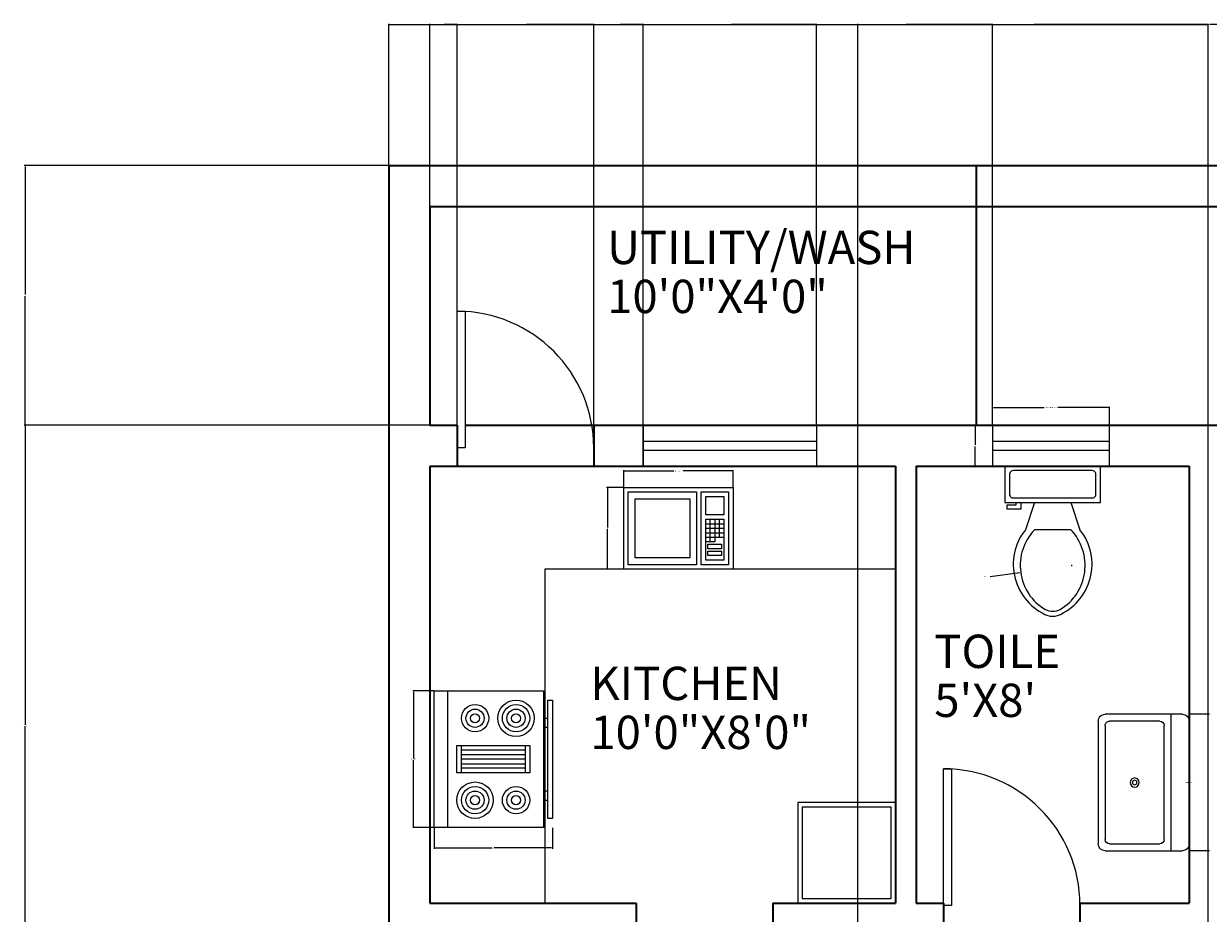
# Model space of a CAD drawing. Units: inches. Extents: x 25018 to 25490, y 41421 to 42101.
# Tile 3 of 5: x 25018 to 25279, y 41906 to 42101. Entities that reach past the tile are written whole.
import ezdxf

# ---------------------------------------------------------------- set-up
doc = ezdxf.new("R2010")
doc.units = ezdxf.units.IN
for name, color, linetype, lineweight in [('A-ANNO-DIMS', 2, 'Continuous', 18), ('A-AREA-IDEN', 7, 'Continuous', 18), ('A-DOOR', 3, 'Continuous', 25), ('A-EQPM', 8, 'Continuous', 18), ('A-FLOR-FIXT', 9, 'Continuous', 18), ('A-GLAZ', 4, 'Continuous', 18), ('A-WALL', 7, 'Continuous', 35)]:
    doc.layers.add(name, color=color, linetype=linetype, lineweight=lineweight)
doc.styles.get("Standard").update_dxf_attribs({"font": 'arial.ttf'})
doc.dimstyles.get("Standard").update_dxf_attribs({"dimtxt": 0.18, "dimasz": 0.18, "dimexe": 0.18, "dimexo": 0.0625, "dimgap": 0.09, "dimtad": 0, "dimtih": 1, "dimtoh": 1, "dimdec": 4, "dimzin": 0, "dimdsep": 46, "dimtxsty": 'Standard', "dimcen": 0.09, "dimadec": 0, "dimazin": 0, "dimtfac": 1, "dimtdec": 4, "dimtofl": 0, "dimtmove": 0, "dimatfit": 3, "dimfxl": 1, "dimtolj": 1, "dimtzin": 0, "dimarcsym": 0})

# ---------------------------------------------------------------- blocks, each defined once
blk = doc.blocks.new('*U2')
for p, q in [((0, 0), (0, -100)), ((750, 0), (750, -100))]:
    blk.add_line(p, q)
blk.add_lwpolyline([(0, 0), (0, 750), (43.75, 750), (43.75, 0)], close=True)
blk.add_arc((0, 0), 750, 0, 90)
blk = doc.blocks.new('Microwave')
for p, q in [((19, 7), (19, 11)), ((20, 11), (20, 7)), ((21, 7), (21, 11)), ((18, 10), (22, 10)), ((22, 9), (18, 9)), ((18, 8), (22, 8)), ((22, 7), (18, 7)), ((20, 6), (18, 6)), ((19, 6), (19, 7)), ((20, 7), (20, 6))]:
    blk.add_line(p, q)
for points in [[(0, 0), (0, 18), (24, 18), (24, 0)], [(1, 1), (1, 17), (16, 17), (16, 1)], [(17, 1), (17, 17), (23, 17), (23, 1)], [(18, 12), (18, 16), (22, 16), (22, 12)], [(2.5, 2.5), (2.5, 15.5), (14.5, 15.5), (14.5, 2.5)], [(18, 2), (18, 11), (22, 11), (22, 2)], [(18.5, 4.5), (18.5, 5.5), (21.5, 5.5), (21.5, 4.5)], [(18.5, 3), (18.5, 4), (21.5, 4), (21.5, 3)]]:
    blk.add_lwpolyline(points, close=True)
blk = doc.blocks.new('Range-Oven - 30 in top')
for p, q in [((0, -3), (30, -3)), ((12, -6), (18, -6)), ((13, -20), (13, -6)), ((14, -6), (14, -20)), ((15, -20), (15, -6)), ((16, -6), (16, -20)), ((17, -20), (17, -6)), ((18, -20), (12, -20)), ((6, -24), (6, -25)), ((8, -25), (8, -24)), ((22, -25), (22, -24)), ((24, -24), (24, -25))]:
    blk.add_line(p, q)
for points in [[(0, -24), (0, 0), (30, 0), (30, -24)], [(12, -21), (12, -5), (18, -5), (18, -21)], [(2, -26), (2, -25), (28, -25), (28, -26)]]:
    blk.add_lwpolyline(points, close=True)
for centre, radius in [((6, -9), 4), ((6, -9), 3), ((6, -9), 2), ((24, -9), 3), ((24, -9), 2), ((6, -9), 1), ((24, -9), 1), ((6, -18), 3), ((24, -18), 4), ((24, -18), 3), ((6, -18), 2), ((6, -18), 1), ((24, -18), 2), ((24, -18), 1)]:
    blk.add_circle(centre, radius)
blk = doc.blocks.new('Toilet - top')
for p, q in [((9.5, -6), (9.5, -2)), ((-10, -8.5), (-8, -8.5)), ((-10, -9.5), (-10, -8.5)), ((-7, -9.5), (-10, -9.5)), ((-8, -8.5), (-8, -8)), ((-7, -8), (-7, -9.5)), ((-4, -8), (-6, -14)), ((4, -8), (6, -14)), ((4, -14), (-4, -14))]:
    blk.add_line(p, q)
blk.add_lwpolyline([(10.5, -8), (10.5, 0), (-10.5, 0), (-10.5, -8)], close=True)
for points in [[(-9.5, -2), (-9.5, -6)], [(8.5, -1), (-8.5, -1)], [(-8.5, -7), (8.5, -7)]]:
    blk.add_lwpolyline(points)
for centre, radius, start, end in [((-8.62, -1.88), 0.884, 81.8699, 188.1301), ((8.62, -1.88), 0.884, 351.8699, 98.1301), ((-8.62, -6.12), 0.884, 171.8699, 278.1301), ((8.62, -6.12), 0.884, 261.8699, 8.1301), ((3.52, -21.58), 12.17, 141.4691, 247.9714), ((4.2, -21.82), 11.33, 136.3677, 238.9468), ((-3.52, -21.58), 12.17, 292.0284, 38.5307), ((-4.2, -21.82), 11.33, 301.053, 43.6321), ((0, -27.88), 4, 245.7318, 294.2682), ((0, -29), 4, 254.8605, 285.1395)]:
    blk.add_arc(centre, radius, start, end)
blk = doc.blocks.new('Sink-single - 30 in top')
blk.add_line((-15, -3.999996), (15, -3.999996))
for points in [[(-13.5, 0), (13.5, 0)], [(-15, -18.499996), (-15, -1.5)], [(15, -1.5), (15, -18.499996)], [(-13.5, -17.499996), (-13.5, -6.499996)], [(-12.5, -5.499996), (12.5, -5.499996)], [(13.5, -6.499996), (13.5, -17.499996)], [(13.5, -19.999996), (-13.5, -19.999996)], [(12.5, -18.499996), (-12.5, -18.499996)]]:
    blk.add_lwpolyline(points)
for radius in [1, 0.5]:
    blk.add_circle((0, -11.999996), radius)
for centre, radius, start, end in [((-13.5, -1.5), 1.5, 90, 180), ((13.5, -1.5), 1.5, 0, 90), ((-12.5, -6.499996), 1, 90, 180), ((12.5, -6.499996), 1, 0, 90), ((-12.5, -17.499996), 1, 180, 270), ((12.5, -17.499996), 1, 270, 0), ((-13.5, -18.499996), 1.5, 180, 270), ((13.5, -18.499996), 1.5, 270, 0)]:
    blk.add_arc(centre, radius, start, end)
blk = doc.blocks.new('WIN-BATH')
for p, q in [((0, 9), (0, 0)), ((25.67, 0), (25.67, 9)), ((0, 5.5), (25.67, 5.5)), ((0, 3.5), (25.67, 3.5))]:
    blk.add_line(p, q)
blk = doc.blocks.new('*D30')
at = {"layer": 'A-ANNO-DIMS', "color": 0, "lineweight": -2, "transparency": 16777216}
for p, q in [((25278.89, 41949.53), (25274.27, 41949.53)), ((25274.45, 41949.35), (25274.45, 41934.71)), ((25274.45, 41919.71), (25274.45, 41934.35)), ((25278.89, 41919.53), (25274.27, 41919.53))]:
    blk.add_line(p, q, dxfattribs=at)
at = {"layer": 'A-ANNO-DIMS', "color": 0, "transparency": 16777216}
for points in [[(25274.42, 41949.35), (25274.48, 41949.35), (25274.45, 41949.53)], [(25274.42, 41919.71), (25274.48, 41919.71), (25274.45, 41919.53)]]:
    blk.add_solid(points, dxfattribs=at)
at = {"layer": 'Defpoints', "color": 0, "transparency": 16777216}
for p in [(25274.45, 41949.53), (25278.95, 41949.53), (25278.95, 41919.53)]:
    blk.add_point(p, dxfattribs=at)
at = {"layer": 'A-ANNO-DIMS', "color": 0, "transparency": 16777216, "insert": (25274.45, 41934.53), "char_height": 0.18, "attachment_point": 5}
blk.add_mtext('\\A1;BASIN 30 TYP.', dxfattribs=at)
blk = doc.blocks.new('*D32')
at = {"layer": 'A-ANNO-DIMS', "color": 0, "lineweight": -2, "transparency": 16777216}
for p, q in [((25231.25, 42013.11), (25231.25, 42017.08)), ((25231.43, 42016.9), (25242.6, 42016.9)), ((25256.74, 42016.9), (25245.57, 42016.9)), ((25256.92, 42013.11), (25256.92, 42017.08))]:
    blk.add_line(p, q, dxfattribs=at)
at = {"layer": 'A-ANNO-DIMS', "color": 0, "transparency": 16777216}
for points in [[(25231.43, 42016.93), (25231.43, 42016.87), (25231.25, 42016.9)], [(25256.74, 42016.93), (25256.74, 42016.87), (25256.92, 42016.9)]]:
    blk.add_solid(points, dxfattribs=at)
at = {"layer": 'Defpoints', "color": 0, "transparency": 16777216}
for p in [(25256.92, 42016.9), (25231.25, 42013.05), (25256.92, 42013.05)]:
    blk.add_point(p, dxfattribs=at)
at = {"layer": 'A-ANNO-DIMS', "color": 0, "transparency": 16777216, "insert": (25244.09, 42016.9), "char_height": 0.18, "attachment_point": 5}
blk.add_mtext('\\A1;BATH WINDOW 26 TYP.', dxfattribs=at)
blk = doc.blocks.new('*D33')
at = {"layer": 'A-ANNO-DIMS', "color": 0, "lineweight": -2, "transparency": 16777216}
for p, q in [((25231.19, 42013.05), (25227.22, 42013.05)), ((25227.4, 42012.87), (25227.4, 42008.73)), ((25227.4, 42004.23), (25227.4, 42008.37)), ((25231.19, 42004.05), (25227.22, 42004.05))]:
    blk.add_line(p, q, dxfattribs=at)
at = {"layer": 'A-ANNO-DIMS', "color": 0, "transparency": 16777216}
for points in [[(25227.37, 42012.87), (25227.43, 42012.87), (25227.4, 42013.05)], [(25227.37, 42004.23), (25227.43, 42004.23), (25227.4, 42004.05)]]:
    blk.add_solid(points, dxfattribs=at)
at = {"layer": 'Defpoints', "color": 0, "transparency": 16777216}
for p in [(25227.4, 42013.05), (25231.25, 42013.05), (25231.25, 42004.05)]:
    blk.add_point(p, dxfattribs=at)
at = {"layer": 'A-ANNO-DIMS', "color": 0, "transparency": 16777216, "insert": (25227.4, 42008.55), "char_height": 0.18, "attachment_point": 5}
blk.add_mtext('\\A1;9 TYP.', dxfattribs=at)
blk = doc.blocks.new('*D34')
at = {"layer": 'A-ANNO-DIMS', "color": 0, "lineweight": -2, "transparency": 16777216}
for p, q in [((25150.25, 41999.43), (25150.25, 42003.15)), ((25150.43, 42002.97), (25161.21, 42002.97)), ((25174.07, 42002.97), (25163.29, 42002.97)), ((25174.25, 41999.43), (25174.25, 42003.15))]:
    blk.add_line(p, q, dxfattribs=at)
at = {"layer": 'A-ANNO-DIMS', "color": 0, "transparency": 16777216}
for points in [[(25150.43, 42003), (25150.43, 42002.94), (25150.25, 42002.97)], [(25174.07, 42003), (25174.07, 42002.94), (25174.25, 42002.97)]]:
    blk.add_solid(points, dxfattribs=at)
at = {"layer": 'Defpoints', "color": 0, "transparency": 16777216}
for p in [(25174.25, 42002.97), (25150.25, 41999.37), (25174.25, 41999.37)]:
    blk.add_point(p, dxfattribs=at)
at = {"layer": 'A-ANNO-DIMS', "color": 0, "transparency": 16777216, "insert": (25162.25, 42002.97), "char_height": 0.18, "attachment_point": 5}
blk.add_mtext('\\A1;MICROWAVE 24', dxfattribs=at)
blk = doc.blocks.new('*D35')
at = {"layer": 'A-ANNO-DIMS', "color": 0, "lineweight": -2, "transparency": 16777216}
for p, q in [((25150.19, 41999.37), (25146.47, 41999.37)), ((25146.65, 41999.19), (25146.65, 41990.55)), ((25146.65, 41981.55), (25146.65, 41990.19)), ((25150.19, 41981.37), (25146.47, 41981.37))]:
    blk.add_line(p, q, dxfattribs=at)
at = {"layer": 'A-ANNO-DIMS', "color": 0, "transparency": 16777216}
for points in [[(25146.62, 41999.19), (25146.68, 41999.19), (25146.65, 41999.37)], [(25146.62, 41981.55), (25146.68, 41981.55), (25146.65, 41981.37)]]:
    blk.add_solid(points, dxfattribs=at)
at = {"layer": 'Defpoints', "color": 0, "transparency": 16777216}
for p in [(25146.65, 41999.37), (25150.25, 41999.37), (25150.25, 41981.37)]:
    blk.add_point(p, dxfattribs=at)
at = {"layer": 'A-ANNO-DIMS', "color": 0, "transparency": 16777216, "insert": (25146.65, 41990.37), "char_height": 0.18, "attachment_point": 5}
blk.add_mtext('\\A1;18', dxfattribs=at)
blk = doc.blocks.new('*D36')
at = {"layer": 'A-ANNO-DIMS', "color": 0, "lineweight": -2, "transparency": 16777216}
for p, q in [((25108.53, 41954.65), (25103.91, 41954.65)), ((25104.09, 41954.47), (25104.09, 41939.84)), ((25104.09, 41924.83), (25104.09, 41939.47)), ((25108.53, 41924.65), (25103.91, 41924.65))]:
    blk.add_line(p, q, dxfattribs=at)
at = {"layer": 'A-ANNO-DIMS', "color": 0, "transparency": 16777216}
for points in [[(25104.06, 41954.47), (25104.12, 41954.47), (25104.09, 41954.65)], [(25104.06, 41924.83), (25104.12, 41924.83), (25104.09, 41924.65)]]:
    blk.add_solid(points, dxfattribs=at)
at = {"layer": 'Defpoints', "color": 0, "transparency": 16777216}
for p in [(25104.09, 41954.65), (25108.59, 41954.65), (25108.59, 41924.65)]:
    blk.add_point(p, dxfattribs=at)
at = {"layer": 'A-ANNO-DIMS', "color": 0, "transparency": 16777216, "insert": (25104.09, 41939.65), "char_height": 0.18, "attachment_point": 5}
blk.add_mtext('\\A1;RANGE 30', dxfattribs=at)
blk = doc.blocks.new('*D37')
at = {"layer": 'A-ANNO-DIMS', "color": 0, "lineweight": -2, "transparency": 16777216}
for p, q in [((25108.59, 41924.59), (25108.59, 41919.97)), ((25134.59, 41924.59), (25134.59, 41919.97)), ((25108.77, 41920.15), (25121.37, 41920.15)), ((25134.41, 41920.15), (25121.81, 41920.15))]:
    blk.add_line(p, q, dxfattribs=at)
at = {"layer": 'A-ANNO-DIMS', "color": 0, "transparency": 16777216}
for points in [[(25108.77, 41920.18), (25108.77, 41920.12), (25108.59, 41920.15)], [(25134.41, 41920.18), (25134.41, 41920.12), (25134.59, 41920.15)]]:
    blk.add_solid(points, dxfattribs=at)
at = {"layer": 'Defpoints', "color": 0, "transparency": 16777216}
for p in [(25108.59, 41924.65), (25134.59, 41924.65), (25108.59, 41920.15)]:
    blk.add_point(p, dxfattribs=at)
at = {"layer": 'A-ANNO-DIMS', "color": 0, "transparency": 16777216, "insert": (25121.59, 41920.15), "char_height": 0.18, "attachment_point": 5}
blk.add_mtext('\\A1;26', dxfattribs=at)
blk = doc.blocks.new('*D38')
at = {"layer": 'A-ANNO-DIMS', "color": 0, "lineweight": -2, "transparency": 16777216}
for p, q in [((25098.65, 42070.11), (25098.65, 42101.23)), ((25098.83, 42101.05), (25278.36, 42101.05)), ((25458.47, 42101.05), (25278.94, 42101.05)), ((25458.65, 42070.11), (25458.65, 42101.23))]:
    blk.add_line(p, q, dxfattribs=at)
at = {"layer": 'A-ANNO-DIMS', "color": 0, "transparency": 16777216}
for points in [[(25098.83, 42101.08), (25098.83, 42101.02), (25098.65, 42101.05)], [(25458.47, 42101.08), (25458.47, 42101.02), (25458.65, 42101.05)]]:
    blk.add_solid(points, dxfattribs=at)
at = {"layer": 'Defpoints', "color": 0, "transparency": 16777216}
for p in [(25458.65, 42101.05), (25098.65, 42070.05), (25458.65, 42070.05)]:
    blk.add_point(p, dxfattribs=at)
at = {"layer": 'A-ANNO-DIMS', "color": 0, "transparency": 16777216, "insert": (25278.65, 42101.05), "char_height": 0.18, "attachment_point": 5}
blk.add_mtext('\\A1;360', dxfattribs=at)
blk = doc.blocks.new('*D48')
at = {"layer": 'A-ANNO-DIMS', "color": 0, "lineweight": -2, "transparency": 16777216}
for p, q in [((25107.59, 42013.05), (25018.58, 42013.05)), ((25018.76, 42012.87), (25018.76, 41947.18)), ((25018.76, 41881.12), (25018.76, 41946.81)), ((25098.59, 41880.94), (25018.58, 41880.94))]:
    blk.add_line(p, q, dxfattribs=at)
at = {"layer": 'A-ANNO-DIMS', "color": 0, "transparency": 16777216}
for points in [[(25018.73, 42012.87), (25018.79, 42012.87), (25018.76, 42013.05)], [(25018.73, 41881.12), (25018.79, 41881.12), (25018.76, 41880.94)]]:
    blk.add_solid(points, dxfattribs=at)
at = {"layer": 'Defpoints', "color": 0, "transparency": 16777216}
for p in [(25018.76, 42013.05), (25107.65, 42013.05), (25098.65, 41880.94)]:
    blk.add_point(p, dxfattribs=at)
at = {"layer": 'A-ANNO-DIMS', "color": 0, "transparency": 16777216, "insert": (25018.76, 41946.99), "char_height": 0.18, "attachment_point": 5}
blk.add_mtext('\\A1;132.1', dxfattribs=at)
blk = doc.blocks.new('*D49')
at = {"layer": 'A-ANNO-DIMS', "color": 0, "lineweight": -2, "transparency": 16777216}
for p, q in [((25098.59, 42070.05), (25018.58, 42070.05)), ((25018.76, 42069.87), (25018.76, 42041.73)), ((25018.76, 42013.23), (25018.76, 42041.37)), ((25107.59, 42013.05), (25018.58, 42013.05))]:
    blk.add_line(p, q, dxfattribs=at)
at = {"layer": 'A-ANNO-DIMS', "color": 0, "transparency": 16777216}
for points in [[(25018.73, 42069.87), (25018.79, 42069.87), (25018.76, 42070.05)], [(25018.73, 42013.23), (25018.79, 42013.23), (25018.76, 42013.05)]]:
    blk.add_solid(points, dxfattribs=at)
at = {"layer": 'Defpoints', "color": 0, "transparency": 16777216}
for p in [(25018.76, 42070.05), (25098.65, 42070.05), (25107.65, 42013.05)]:
    blk.add_point(p, dxfattribs=at)
at = {"layer": 'A-ANNO-DIMS', "color": 0, "transparency": 16777216, "insert": (25018.76, 42041.55), "char_height": 0.18, "attachment_point": 5}
blk.add_mtext('\\A1;57', dxfattribs=at)
blk = doc.blocks.new('*D59')
at = {"layer": 'A-ANNO-DIMS', "color": 0, "lineweight": -2, "transparency": 16777216}
for p, q in [((25107.652612, 42013.112335), (25107.652612, 42101.229835)), ((25107.832612, 42101.049835), (25110.503185, 42101.049835)), ((25113.472612, 42101.049835), (25110.802039, 42101.049835)), ((25113.652612, 42013.112335), (25113.652612, 42101.229835))]:
    blk.add_line(p, q, dxfattribs=at)
at = {"layer": 'A-ANNO-DIMS', "color": 0, "transparency": 16777216}
for points in [[(25107.832612, 42101.079835), (25107.832612, 42101.019835), (25107.652612, 42101.049835)], [(25113.472612, 42101.079835), (25113.472612, 42101.019835), (25113.652612, 42101.049835)]]:
    blk.add_solid(points, dxfattribs=at)
at = {"layer": 'Defpoints', "color": 0, "transparency": 16777216}
for p in [(25113.652612, 42101.049835), (25107.652612, 42013.049835), (25113.652612, 42013.049835)]:
    blk.add_point(p, dxfattribs=at)
at = {"layer": 'A-ANNO-DIMS', "color": 0, "transparency": 16777216, "insert": (25110.652612, 42101.049835), "char_height": 0.18, "attachment_point": 5}
blk.add_mtext('\\A1;6', dxfattribs=at)
blk = doc.blocks.new('*D60')
at = {"layer": 'A-ANNO-DIMS', "color": 0, "lineweight": -2, "transparency": 16777216}
for p, q in [((25113.65, 42013.11), (25113.65, 42101.23)), ((25113.83, 42101.05), (25128.43, 42101.05)), ((25143.47, 42101.05), (25128.87, 42101.05)), ((25143.65, 42013.11), (25143.65, 42101.23))]:
    blk.add_line(p, q, dxfattribs=at)
at = {"layer": 'A-ANNO-DIMS', "color": 0, "transparency": 16777216}
for points in [[(25113.83, 42101.08), (25113.83, 42101.02), (25113.65, 42101.05)], [(25143.47, 42101.08), (25143.47, 42101.02), (25143.65, 42101.05)]]:
    blk.add_solid(points, dxfattribs=at)
at = {"layer": 'Defpoints', "color": 0, "transparency": 16777216}
for p in [(25143.65, 42101.05), (25113.65, 42013.05), (25143.65, 42013.05)]:
    blk.add_point(p, dxfattribs=at)
at = {"layer": 'A-ANNO-DIMS', "color": 0, "transparency": 16777216, "insert": (25128.65, 42101.05), "char_height": 0.18, "attachment_point": 5}
blk.add_mtext('\\A1;30', dxfattribs=at)
blk = doc.blocks.new('*D61')
at = {"layer": 'A-ANNO-DIMS', "color": 0, "lineweight": -2, "transparency": 16777216}
for p, q in [((25143.65, 42013.11), (25143.65, 42101.23)), ((25143.83, 42101.05), (25148.62, 42101.05)), ((25154.32, 42101.05), (25149.53, 42101.05)), ((25154.5, 42013.11), (25154.5, 42101.23))]:
    blk.add_line(p, q, dxfattribs=at)
at = {"layer": 'A-ANNO-DIMS', "color": 0, "transparency": 16777216}
for points in [[(25143.83, 42101.08), (25143.83, 42101.02), (25143.65, 42101.05)], [(25154.32, 42101.08), (25154.32, 42101.02), (25154.5, 42101.05)]]:
    blk.add_solid(points, dxfattribs=at)
at = {"layer": 'Defpoints', "color": 0, "transparency": 16777216}
for p in [(25154.5, 42101.05), (25143.65, 42013.05), (25154.5, 42013.05)]:
    blk.add_point(p, dxfattribs=at)
at = {"layer": 'A-ANNO-DIMS', "color": 0, "transparency": 16777216, "insert": (25149.08, 42101.05), "char_height": 0.18, "attachment_point": 5}
blk.add_mtext('\\A1;10.849', dxfattribs=at)
blk = doc.blocks.new('*D62')
at = {"layer": 'A-ANNO-DIMS', "color": 0, "lineweight": -2, "transparency": 16777216}
for p, q in [((25154.5, 42013.11), (25154.5, 42101.23)), ((25154.68, 42101.05), (25173.14, 42101.05)), ((25192.38, 42101.05), (25173.93, 42101.05)), ((25192.56, 42013.11), (25192.56, 42101.23))]:
    blk.add_line(p, q, dxfattribs=at)
at = {"layer": 'A-ANNO-DIMS', "color": 0, "transparency": 16777216}
for points in [[(25154.68, 42101.08), (25154.68, 42101.02), (25154.5, 42101.05)], [(25192.38, 42101.08), (25192.38, 42101.02), (25192.56, 42101.05)]]:
    blk.add_solid(points, dxfattribs=at)
at = {"layer": 'Defpoints', "color": 0, "transparency": 16777216}
for p in [(25192.56, 42101.05), (25154.5, 42013.05), (25192.56, 42013.05)]:
    blk.add_point(p, dxfattribs=at)
at = {"layer": 'A-ANNO-DIMS', "color": 0, "transparency": 16777216, "insert": (25173.53, 42101.05), "char_height": 0.18, "attachment_point": 5}
blk.add_mtext('\\A1;38.06', dxfattribs=at)
blk = doc.blocks.new('*D63')
at = {"layer": 'A-ANNO-DIMS', "color": 0, "lineweight": -2, "transparency": 16777216}
for p, q in [((25192.56, 42013.11), (25192.56, 42101.23)), ((25192.74, 42101.05), (25211.51, 42101.05)), ((25231.07, 42101.05), (25212.3, 42101.05)), ((25231.25, 42013.11), (25231.25, 42101.23))]:
    blk.add_line(p, q, dxfattribs=at)
at = {"layer": 'A-ANNO-DIMS', "color": 0, "transparency": 16777216}
for points in [[(25192.74, 42101.08), (25192.74, 42101.02), (25192.56, 42101.05)], [(25231.07, 42101.08), (25231.07, 42101.02), (25231.25, 42101.05)]]:
    blk.add_solid(points, dxfattribs=at)
at = {"layer": 'Defpoints', "color": 0, "transparency": 16777216}
for p in [(25231.25, 42101.05), (25192.56, 42013.05), (25231.25, 42013.05)]:
    blk.add_point(p, dxfattribs=at)
at = {"layer": 'A-ANNO-DIMS', "color": 0, "transparency": 16777216, "insert": (25211.91, 42101.05), "char_height": 0.18, "attachment_point": 5}
blk.add_mtext('\\A1;38.69', dxfattribs=at)
blk = doc.blocks.new('*D75')
at = {"layer": 'A-ANNO-DIMS', "color": 0, "lineweight": -2, "transparency": 16777216}
for p, q in [((25201.64, 41804.94), (25201.64, 42101.23)), ((25201.82, 42101.05), (25239.92, 42101.05)), ((25278.45, 42101.05), (25240.36, 42101.05)), ((25278.63, 41804.94), (25278.63, 42101.23))]:
    blk.add_line(p, q, dxfattribs=at)
at = {"layer": 'A-ANNO-DIMS', "color": 0, "transparency": 16777216}
for points in [[(25201.82, 42101.08), (25201.82, 42101.02), (25201.64, 42101.05)], [(25278.45, 42101.08), (25278.45, 42101.02), (25278.63, 42101.05)]]:
    blk.add_solid(points, dxfattribs=at)
at = {"layer": 'Defpoints', "color": 0, "transparency": 16777216}
for p in [(25278.63, 42101.05), (25201.64, 41804.88), (25278.63, 41804.88)]:
    blk.add_point(p, dxfattribs=at)
at = {"layer": 'A-ANNO-DIMS', "color": 0, "transparency": 16777216, "insert": (25240.14, 42101.05), "char_height": 0.18, "attachment_point": 5}
blk.add_mtext('\\A1;77', dxfattribs=at)
blk = doc.blocks.new('*D79')
at = {"layer": 'A-ANNO-DIMS', "color": 0, "lineweight": -2, "transparency": 16777216}
for p, q in [((25230.69, 41979.82), (25237.25, 41980.7)), ((25248.56, 41982.23), (25248.74, 41982.23)), ((25248.65, 41982.14), (25248.65, 41982.32))]:
    blk.add_line(p, q, dxfattribs=at)
at = {"layer": 'A-ANNO-DIMS', "color": 0, "transparency": 16777216}
blk.add_solid([(25237.24, 41980.73), (25237.25, 41980.67), (25237.42, 41980.72)], dxfattribs=at)
at = {"layer": 'Defpoints', "color": 0, "transparency": 16777216}
for p in [(25237.42, 41980.72), (25248.65, 41982.23)]:
    blk.add_point(p, dxfattribs=at)
at = {"layer": 'A-ANNO-DIMS', "color": 0, "transparency": 16777216, "insert": (25230.01, 41979.82), "char_height": 0.18, "attachment_point": 5}
blk.add_mtext('\\A1;4X R11.33', dxfattribs=at)

msp = doc.modelspace()

# ---------------------------------------------------------------- linework, layer by layer
at = {"layer": 'A-FLOR-FIXT'}
for p, q in [((25209.9527, 41981.3695), (25132.9429, 41981.3695)), ((25132.9429, 41981.3695), (25132.9429, 41908.0498))]:
    msp.add_line(p, q, dxfattribs=at)
for points in [[(25188.4523, 41908.0498), (25209.9527, 41908.0498), (25209.9527, 41930.1447), (25188.4523, 41930.1447)], [(25189.4523, 41909.0498), (25208.9527, 41909.0498), (25208.9527, 41929.1447), (25189.4523, 41929.1447)]]:
    msp.add_lwpolyline(points, close=True, dxfattribs=at)
at = {"layer": 'A-GLAZ'}
for p, q in [((25192.5647, 42013.0498), (25192.5647, 42004.0498)), ((25154.5013, 42009.5498), (25192.5647, 42009.5498)), ((25154.5013, 42007.5498), (25192.5647, 42007.5498))]:
    msp.add_line(p, q, dxfattribs=at)
msp.add_lwpolyline([(25154.5013, 42013.0498), (25154.5013, 42013.0498), (25154.5013, 42004.0498), (25154.5013, 42004.0498)], close=True, dxfattribs=at)
at = {"layer": 'A-WALL'}
for p, q in [((25098.6526, 42070.0498), (25458.6526, 42070.0498)), ((25098.6526, 42070.0498), (25098.6526, 41501.5498)), ((25227.6526, 42070.0498), (25227.6526, 42013.0498)), ((25107.6526, 42061.0498), (25449.6526, 42061.0498)), ((25107.6526, 42061.0498), (25107.6526, 42013.0498)), ((25107.6526, 42013.0498), (25113.6526, 42013.0498)), ((25113.6526, 42013.0498), (25113.6526, 42004.0498)), ((25115.4026, 42013.0498), (25449.6526, 42013.0498)), ((25143.6526, 42013.0498), (25143.6526, 42004.0498)), ((25107.6526, 42004.0498), (25113.6526, 42004.0498)), ((25107.6526, 42004.0498), (25107.6526, 41908.0498)), ((25113.6526, 42004.0498), (25209.9527, 42004.0498)), ((25209.9527, 42004.0498), (25209.9527, 41908.0498)), ((25214.4527, 42004.0498), (25214.4527, 41908.0498)), ((25214.4527, 42004.0498), (25274.4527, 42004.0498)), ((25274.4527, 42004.0498), (25274.4527, 41908.0498)), ((25107.6526, 41908.0498), (25152.9888, 41908.0498)), ((25152.9888, 41908.0498), (25152.9888, 41903.5498)), ((25182.9888, 41908.0498), (25182.9888, 41903.5498)), ((25182.9888, 41908.0498), (25209.9527, 41908.0498)), ((25214.4527, 41908.0498), (25220.4527, 41908.0498)), ((25220.4527, 41908.0498), (25220.4527, 41903.5498)), ((25250.4527, 41908.0498), (25250.4527, 41903.5498)), ((25250.4527, 41908.0498), (25274.4527, 41908.0498))]:
    msp.add_line(p, q, dxfattribs=at)

# ---------------------------------------------------------------- block references
at = {"layer": 'A-DOOR', "xscale": 0.0400000000000011, "yscale": 0.0400000000000011, "zscale": 0.0400000000000011}
for p in [(25113.6526, 42008.0498), (25220.4527, 41907.5498)]:
    msp.add_blockref('*U2', p, dxfattribs=at)
at = {"layer": 'A-EQPM'}
msp.add_blockref('Microwave', (25150.248, 41981.3695), dxfattribs=at)
at = {"layer": 'A-EQPM', "rotation": 90}
msp.add_blockref('Range-Oven - 30 in top', (25108.5882, 41924.6525), dxfattribs=at)
at = {"layer": 'A-FLOR-FIXT'}
msp.add_blockref('Toilet - top', (25244.4527, 42004.0498), dxfattribs=at)
at = {"layer": 'A-FLOR-FIXT', "xscale": -1, "rotation": 270}
msp.add_blockref('Sink-single - 30 in top', (25274.4527, 41934.5291), dxfattribs=at)
at = {"layer": 'A-GLAZ'}
msp.add_blockref('WIN-BATH', (25231.251, 42004.05), dxfattribs=at)

# ---------------------------------------------------------------- texts
at = {"layer": 'A-AREA-IDEN'}
for s, height, p in [('UTILITY/WASH', 7.320471, (25146.599, 42048.423)), ('10\'0"X4\'0"', 7.32047, (25146.6067, 42037.6638)), ('TOILE', 7.32047, (25218.446, 41959.6927)), ('KITCHEN', 7.32047, (25142.9083, 41952.6525)), ("5'X8'", 7.32047, (25218.4536, 41948.9335)), ('10\'0"X8\'0"', 7.32047, (25142.9159, 41941.8932))]:
    msp.add_text(s, height=height, dxfattribs=at).set_placement(p)

# ---------------------------------------------------------------- dimensions: what is measured, and where the dimension line sits
at = {"layer": 'A-ANNO-DIMS'}
for base, p1, p2, override, picture, middle in [((25458.6526, 42101.0498), (25098.6526, 42070.0498), (25458.6526, 42070.0498), {"dimdec": 0, "dimlfac": 1, "dimrnd": 0, "dimzin": 0, "dimdsep": 46, "dimlunit": 2}, '*D38', (25278.6526, 42101.0498)), ((25113.6526, 42101.0498), (25107.6526, 42013.0498), (25113.6526, 42013.0498), {"dimdec": 0, "dimlfac": 1, "dimrnd": 0, "dimzin": 0, "dimdsep": 46, "dimlunit": 2}, '*D59', (25110.6526, 42101.0498)), ((25143.6526, 42101.0498), (25113.6526, 42013.0498), (25143.6526, 42013.0498), {"dimdec": 0, "dimlfac": 1, "dimrnd": 0, "dimzin": 0, "dimdsep": 46, "dimlunit": 2}, '*D60', (25128.6526, 42101.0498)), ((25154.5013, 42101.0498), (25143.6526, 42013.0498), (25154.5013, 42013.0498), {"dimdec": 3, "dimlfac": 1, "dimrnd": 0, "dimzin": 0, "dimdsep": 46, "dimlunit": 2}, '*D61', (25149.077, 42101.0498)), ((25192.5647, 42101.0498), (25154.5013, 42013.0498), (25192.5647, 42013.0498), {"dimdec": 2, "dimlfac": 1, "dimrnd": 0, "dimzin": 0, "dimdsep": 46, "dimlunit": 2}, '*D62', (25173.533, 42101.0498)), ((25231.251, 42101.0498), (25192.5647, 42013.0498), (25231.251, 42013.0498), {"dimdec": 2, "dimlfac": 1, "dimrnd": 0, "dimzin": 0, "dimdsep": 46, "dimlunit": 2}, '*D63', (25211.9078, 42101.0498)), ((25278.6341, 42101.0498), (25201.6418, 41804.8791), (25278.6341, 41804.8791), {"dimdec": 0, "dimlfac": 1, "dimrnd": 0, "dimzin": 0, "dimdsep": 46, "dimlunit": 2}, '*D75', (25240.138, 42101.0498))]:
    dim = msp.add_linear_dim(base=base, p1=p1, p2=p2, dimstyle='Standard', override=override, dxfattribs=at)
    dim.commit()
    dim.dimension.update_dxf_attribs({"geometry": picture, "text_midpoint": middle})
for base, p1, p2, angle, override, picture, middle in [((25018.7568, 42070.0498), (25107.6526, 42013.0498), (25098.6526, 42070.0498), 90, {"dimdec": 0, "dimlfac": 1, "dimrnd": 0, "dimzin": 0, "dimdsep": 46, "dimlunit": 2}, '*D49', (25018.7568, 42041.5498)), ((25018.7568, 42013.0498), (25098.6526, 41880.9383), (25107.6526, 42013.0498), 90, {"dimdec": 1, "dimlfac": 1, "dimrnd": 0, "dimzin": 0, "dimdsep": 46, "dimlunit": 2}, '*D48', (25018.7568, 41946.994)), ((25146.648, 41999.3695), (25150.248, 41981.3695), (25150.248, 41999.3695), 90, {"dimdec": 0, "dimlfac": 1, "dimrnd": 0, "dimzin": 0, "dimdsep": 46, "dimlunit": 2}, '*D35', (25146.648, 41990.3695)), ((25108.5882, 41920.1525), (25134.5882, 41924.6525), (25108.5882, 41924.6525), 180, {"dimdec": 0, "dimlfac": 1, "dimrnd": 0, "dimzin": 0, "dimdsep": 46, "dimlunit": 2}, '*D37', (25121.5882, 41920.1525))]:
    dim = msp.add_linear_dim(base=base, p1=p1, p2=p2, angle=angle, dimstyle='Standard', override=override, dxfattribs=at)
    dim.commit()
    dim.dimension.update_dxf_attribs({"geometry": picture, "text_midpoint": middle})
for base, p1, p2, text, picture, middle in [((25256.9199, 42016.9002), (25231.251, 42013.0498), (25256.9199, 42013.0498), 'BATH WINDOW <> TYP.', '*D32', (25244.0854, 42016.9002)), ((25174.248, 42002.9695), (25150.248, 41999.3695), (25174.248, 41999.3695), 'MICROWAVE <>', '*D34', (25162.248, 42002.9695))]:
    dim = msp.add_linear_dim(base=base, p1=p1, p2=p2, text=text, dimstyle='Standard', override={"dimdec": 0, "dimlfac": 1, "dimrnd": 0, "dimzin": 0, "dimdsep": 46, "dimlunit": 2}, dxfattribs=at)
    dim.commit()
    dim.dimension.update_dxf_attribs({"geometry": picture, "text_midpoint": middle})
for base, p1, p2, text, picture, middle in [((25227.4006, 42013.0498), (25231.251, 42004.0498), (25231.251, 42013.0498), '<> TYP.', '*D33', (25227.4006, 42008.5498)), ((25104.0882, 41954.6525), (25108.5882, 41924.6525), (25108.5882, 41954.6525), 'RANGE <>', '*D36', (25104.0882, 41939.6525)), ((25274.4527, 41949.5291), (25278.9527, 41919.5291), (25278.9527, 41949.5291), 'BASIN <> TYP.', '*D30', (25274.4527, 41934.5291))]:
    dim = msp.add_linear_dim(base=base, p1=p1, p2=p2, angle=90, text=text, dimstyle='Standard', override={"dimdec": 0, "dimlfac": 1, "dimrnd": 0, "dimzin": 0, "dimdsep": 46, "dimlunit": 2}, dxfattribs=at)
    dim.commit()
    dim.dimension.update_dxf_attribs({"geometry": picture, "text_midpoint": middle})
dim = msp.add_radius_dim(center=(25248.6527, 41982.2324), mpoint=(25237.4245, 41980.7229), text='4X <>', dimstyle='Standard', override={"dimdec": 2, "dimlfac": 1, "dimrnd": 0, "dimzin": 0, "dimdsep": 46, "dimlunit": 2}, dxfattribs=at)
dim.commit()
dim.dimension.update_dxf_attribs({"geometry": '*D79', "text_midpoint": (25230.6876, 41979.8172), "dimtype": 164})

doc.saveas('drawing.dxf')
